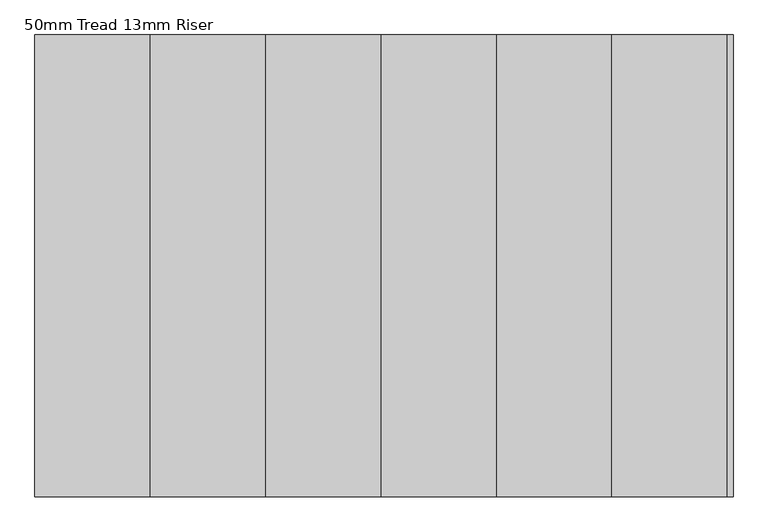
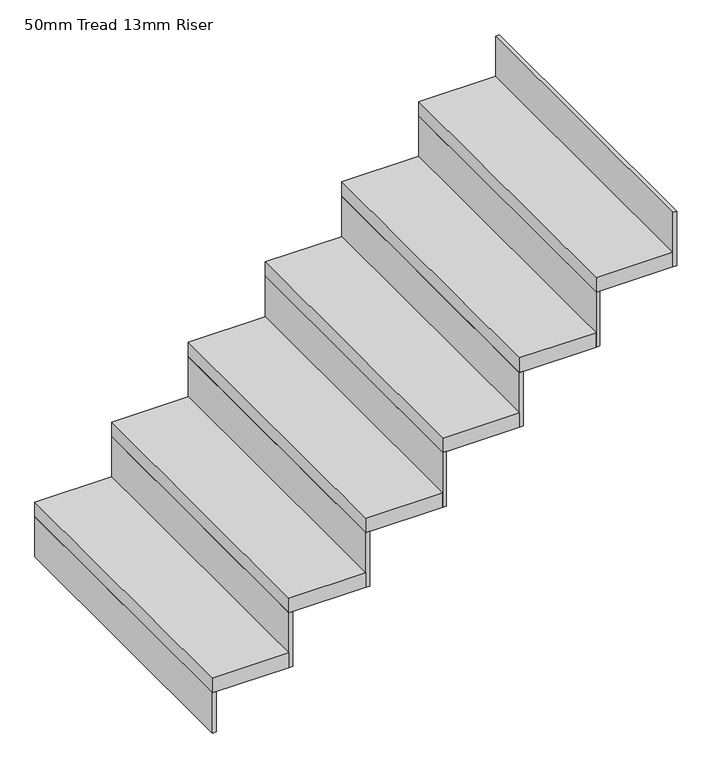
"""IFC4 building model written with IfcOpenShell, lengths in millimetres: stair flight geometry, 50mm Tread 13mm Riser."""

from ifc_helpers import new_model, si_unit, frame, origin, place, context, project, spatial, polyline, outline, extrude, source, transform, mapped, element, save


def stair_flight_50mm_tread_13mm_riser_d6021486(model_context):
    return source(origin(), model_context, "Body", "SweptSolid", [
        extrude(outline(polyline([(-11979.6794909, -2507.9876321), (-11992.1794909, -2507.9876321), (-11992.1794909, -1507.9618509), (-11979.6794909, -1507.9618509), (-11979.6794909, -2507.9876321)])), frame((0.0, 0.0, 9601.2), z_axis=(0.0, 0.0, 1.0), x_axis=(1.0, 0.0, 0.0)), (0.0, 0.0, 1.0), 138.2588235),
        extrude(outline(polyline([(-11742.1794909, -1507.9618509), (-11742.1794909, -2507.9876321), (-11992.1794909, -2507.9876321), (-11992.1794909, -1507.9618509), (-11742.1794909, -1507.9618509)])), frame((0.0, 0.0, 9739.4588235), z_axis=(0.0, 0.0, 1.0), x_axis=(1.0, 0.0, 0.0)), (0.0, 0.0, 1.0), 50.0),
        extrude(outline(polyline([(-11729.6794909, -2507.9876321), (-11742.1794909, -2507.9876321), (-11742.1794909, -1507.9618509), (-11729.6794909, -1507.9618509), (-11729.6794909, -2507.9876321)])), frame((0.0, 0.0, 9739.4588235), z_axis=(0.0, 0.0, 1.0), x_axis=(1.0, 0.0, 0.0)), (0.0, 0.0, 1.0), 188.2588235),
        extrude(outline(polyline([(-11492.1794909, -1507.9618509), (-11492.1794909, -2507.9876321), (-11742.1794909, -2507.9876321), (-11742.1794909, -1507.9618509), (-11492.1794909, -1507.9618509)])), frame((0.0, 0.0, 9927.7176471), z_axis=(0.0, 0.0, 1.0), x_axis=(1.0, 0.0, 0.0)), (0.0, 0.0, 1.0), 50.0),
        extrude(outline(polyline([(-11479.6794909, -2507.9876321), (-11492.1794909, -2507.9876321), (-11492.1794909, -1507.9618509), (-11479.6794909, -1507.9618509), (-11479.6794909, -2507.9876321)])), frame((0.0, 0.0, 9927.7176471), z_axis=(0.0, 0.0, 1.0), x_axis=(1.0, 0.0, 0.0)), (0.0, 0.0, 1.0), 188.2588235),
        extrude(outline(polyline([(-11242.1794909, -1507.9618509), (-11242.1794909, -2507.9876321), (-11492.1794909, -2507.9876321), (-11492.1794909, -1507.9618509), (-11242.1794909, -1507.9618509)])), frame((0.0, 0.0, 10115.9764706), z_axis=(0.0, 0.0, 1.0), x_axis=(1.0, 0.0, 0.0)), (0.0, 0.0, 1.0), 50.0),
        extrude(outline(polyline([(-11229.6794909, -2507.9876321), (-11242.1794909, -2507.9876321), (-11242.1794909, -1507.9618509), (-11229.6794909, -1507.9618509), (-11229.6794909, -2507.9876321)])), frame((0.0, 0.0, 10115.9764706), z_axis=(0.0, 0.0, 1.0), x_axis=(1.0, 0.0, 0.0)), (0.0, 0.0, 1.0), 188.2588235),
        extrude(outline(polyline([(-10992.1794909, -1507.9618509), (-10992.1794909, -2507.9876321), (-11242.1794909, -2507.9876321), (-11242.1794909, -1507.9618509), (-10992.1794909, -1507.9618509)])), frame((0.0, 0.0, 10304.2352941), z_axis=(0.0, 0.0, 1.0), x_axis=(1.0, 0.0, 0.0)), (0.0, 0.0, 1.0), 50.0),
        extrude(outline(polyline([(-10979.6794909, -2507.9876321), (-10992.1794909, -2507.9876321), (-10992.1794909, -1507.9618509), (-10979.6794909, -1507.9618509), (-10979.6794909, -2507.9876321)])), frame((0.0, 0.0, 10304.2352941), z_axis=(0.0, 0.0, 1.0), x_axis=(1.0, 0.0, 0.0)), (0.0, 0.0, 1.0), 188.2588235),
        extrude(outline(polyline([(-10742.1794909, -1507.9618509), (-10742.1794909, -2507.9876321), (-10992.1794909, -2507.9876321), (-10992.1794909, -1507.9618509), (-10742.1794909, -1507.9618509)])), frame((0.0, 0.0, 10492.4941176), z_axis=(0.0, 0.0, 1.0), x_axis=(1.0, 0.0, 0.0)), (0.0, 0.0, 1.0), 50.0),
        extrude(outline(polyline([(-10729.6794909, -2507.9876321), (-10742.1794909, -2507.9876321), (-10742.1794909, -1507.9618509), (-10729.6794909, -1507.9618509), (-10729.6794909, -2507.9876321)])), frame((0.0, 0.0, 10492.4941176), z_axis=(0.0, 0.0, 1.0), x_axis=(1.0, 0.0, 0.0)), (0.0, 0.0, 1.0), 188.2588235),
        extrude(outline(polyline([(-10479.6794909, -2507.9876321), (-10492.1794909, -2507.9876321), (-10492.1794909, -1507.9618509), (-10479.6794909, -1507.9618509), (-10479.6794909, -2507.9876321)])), frame((0.0, 0.0, 10680.7529412), z_axis=(0.0, 0.0, 1.0), x_axis=(1.0, 0.0, 0.0)), (0.0, 0.0, 1.0), 188.2588235),
        extrude(outline(polyline([(-10492.1794909, -1507.9618509), (-10492.1794909, -2507.9876321), (-10742.1794909, -2507.9876321), (-10742.1794909, -1507.9618509), (-10492.1794909, -1507.9618509)])), frame((0.0, 0.0, 10680.7529412), z_axis=(0.0, 0.0, 1.0), x_axis=(1.0, 0.0, 0.0)), (0.0, 0.0, 1.0), 50.0),
    ])


if __name__ == "__main__":
    model = new_model("IFC4")
    model_context = context("Model", 3, world=origin())
    ifc_project = project(units=[si_unit("LENGTHUNIT", "METRE", prefix="MILLI")], contexts=[model_context])
    site = spatial("IfcSite", under=ifc_project)
    building = spatial("IfcBuilding", under=site)
    placement = place(None, origin())
    stair_flight_50mm_tread_13mm_riser_shape = stair_flight_50mm_tread_13mm_riser_d6021486(model_context)
    element("IfcStairFlight", 1, ObjectType="50mm Tread 13mm Riser", at=placement, inside=building, context=model_context, shape_type="MappedRepresentation", body=[
        mapped(stair_flight_50mm_tread_13mm_riser_shape, transform((0.0, 0.0, 0.0), x_axis=(1.0, 0.0, 0.0), y_axis=(0.0, 1.0, 0.0), z_axis=(0.0, 0.0, 1.0))),
    ])
    save(model, "model.ifc")
